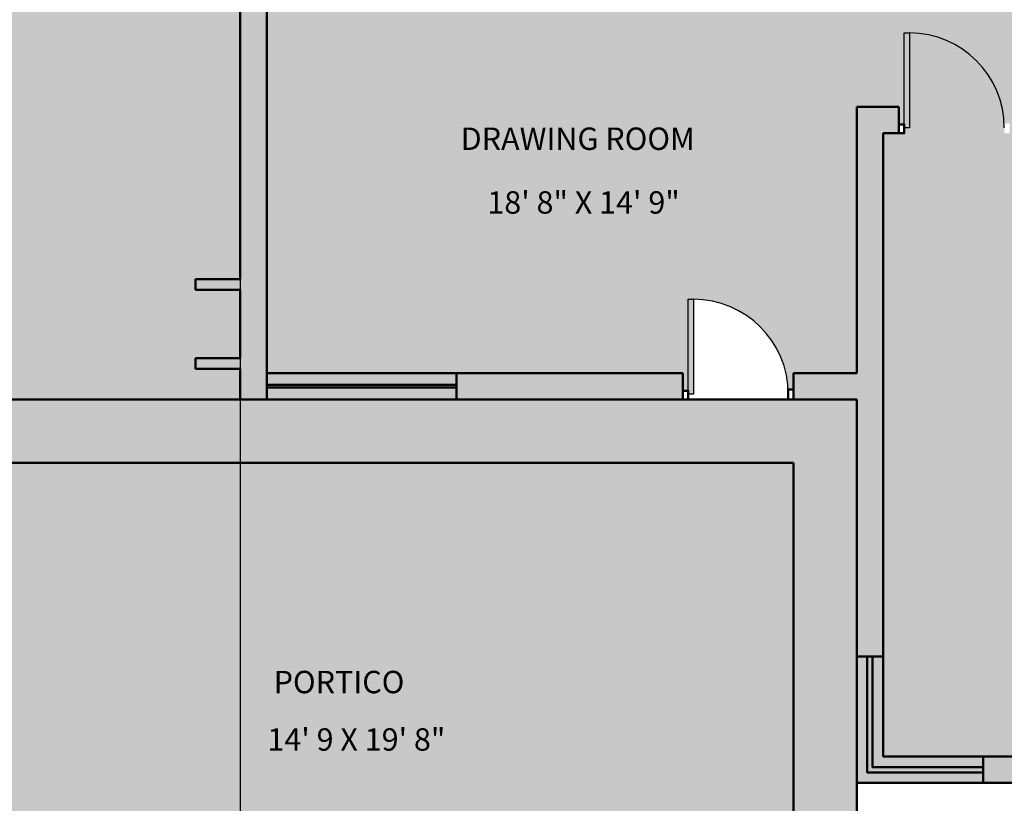
# Model space of a CAD drawing. Units: inches. Extents: x 925 to 2834, y 111 to 1355.
# Tile 3 of 25: x 1116 to 1490, y 377 to 675. Entities that reach past the tile are written whole.
import ezdxf

# ---------------------------------------------------------------- set-up
doc = ezdxf.new("R2010")
doc.units = ezdxf.units.IN
doc.header["$MEASUREMENT"] = 0
for name, color, linetype, lineweight in [('A-ANNO-DIMS', 2, 'Continuous', 18), ('A-AREA-IDEN', 7, 'Continuous', 18), ('A-DOOR', 2, 'Continuous', 25), ('A-FLOR-PATT', 252, 'Continuous', 13), ('A-WALL', 7, 'Continuous', 50), ('A-WALL-PATT', 8, 'Continuous', 13)]:
    doc.layers.add(name, color=color, linetype=linetype, lineweight=lineweight)
doc.styles.get("Standard").update_dxf_attribs({"font": 'arial.ttf'})
doc.dimstyles.get("Standard").update_dxf_attribs({"dimtxt": 6, "dimasz": 3, "dimexe": 0.18, "dimexo": 0.0625, "dimgap": 0.09, "dimtad": 0, "dimtih": 1, "dimtoh": 1, "dimdec": 1, "dimzin": 0, "dimdsep": 46, "dimlunit": 3, "dimtxsty": 'Standard', "dimblk": 'ARCHTICK', "dimcen": 0.09, "dimadec": 0, "dimazin": 0, "dimtfac": 1, "dimtdec": 1, "dimtofl": 0, "dimtmove": 0, "dimatfit": 3, "dimfxl": 1, "dimtolj": 1, "dimtzin": 0, "dimarcsym": 0})

# ---------------------------------------------------------------- blocks, each defined once
blk = doc.blocks.new('DOOR-900')
for p, q in [((0, 0), (0, 36)), ((0, 36), (2, 36)), ((2, 36), (2, 0)), ((2, 0), (0, 0))]:
    blk.add_line(p, q)
blk.add_arc((2, 0), 36, 0, 90)
blk = doc.blocks.new('_ArchTick')
at = {"color": 0, "linetype": 'ByBlock', "const_width": 0.15}
blk.add_lwpolyline([(-0.5, -0.5), (0.5, 0.5)], dxfattribs=at)
blk = doc.blocks.new('*D25')
at = {"layer": 'A-ANNO-DIMS', "color": 0, "lineweight": -2, "transparency": 16777216}
for p, q in [((1200.21, 727.53), (1200.21, 115.18)), ((1084.71, 265.03), (1084.71, 115.18)), ((1084.71, 115.36), (1132.51, 115.36)), ((1200.21, 115.36), (1152.42, 115.36))]:
    blk.add_line(p, q, dxfattribs=at)
at = {"layer": 'Defpoints', "color": 0, "transparency": 16777216}
for p in [(1200.21, 727.59), (1084.71, 265.09), (1200.21, 115.36)]:
    blk.add_point(p, dxfattribs=at)
at = {"layer": 'A-ANNO-DIMS', "color": 0, "lineweight": -2, "transparency": 16777216, "xscale": 3, "yscale": 3, "zscale": 3, "rotation": 180}
blk.add_blockref('_ArchTick', (1084.71, 115.36), dxfattribs=at)
at = {"layer": 'A-ANNO-DIMS', "color": 0, "lineweight": -2, "transparency": 16777216, "xscale": 3, "yscale": 3, "zscale": 3}
blk.add_blockref('_ArchTick', (1200.21, 115.36), dxfattribs=at)
at = {"layer": 'A-ANNO-DIMS', "color": 0, "transparency": 16777216, "insert": (1142.46, 115.36), "char_height": 6, "attachment_point": 5}
blk.add_mtext('\\A1;115.5', dxfattribs=at)
blk = doc.blocks.new('*D26')
at = {"layer": 'A-ANNO-DIMS', "color": 0, "lineweight": -2, "transparency": 16777216}
for p, q in [((1200.21, 727.53), (1200.21, 115.18)), ((1434.21, 385.03), (1434.21, 115.18)), ((1200.21, 115.36), (1310.46, 115.36)), ((1434.21, 115.36), (1323.97, 115.36))]:
    blk.add_line(p, q, dxfattribs=at)
at = {"layer": 'Defpoints', "color": 0, "transparency": 16777216}
for p in [(1200.21, 727.59), (1434.21, 385.09), (1434.21, 115.36)]:
    blk.add_point(p, dxfattribs=at)
at = {"layer": 'A-ANNO-DIMS', "color": 0, "lineweight": -2, "transparency": 16777216, "xscale": 3, "yscale": 3, "zscale": 3, "rotation": 180}
blk.add_blockref('_ArchTick', (1200.21, 115.36), dxfattribs=at)
at = {"layer": 'A-ANNO-DIMS', "color": 0, "lineweight": -2, "transparency": 16777216, "xscale": 3, "yscale": 3, "zscale": 3}
blk.add_blockref('_ArchTick', (1434.21, 115.36), dxfattribs=at)
at = {"layer": 'A-ANNO-DIMS', "color": 0, "transparency": 16777216, "insert": (1317.21, 115.36), "char_height": 6, "attachment_point": 5}
blk.add_mtext('\\A1;234', dxfattribs=at)
blk = doc.blocks.new('*D27')
at = {"layer": 'A-ANNO-DIMS', "color": 0, "lineweight": -2, "transparency": 16777216}
for p, q in [((1621.21, 395.03), (1621.21, 115.18)), ((1434.21, 385.03), (1434.21, 115.18)), ((1434.21, 115.36), (1521.28, 115.36)), ((1621.21, 115.36), (1534.15, 115.36))]:
    blk.add_line(p, q, dxfattribs=at)
at = {"layer": 'Defpoints', "color": 0, "transparency": 16777216}
for p in [(1621.21, 395.09), (1434.21, 385.09), (1621.21, 115.36)]:
    blk.add_point(p, dxfattribs=at)
at = {"layer": 'A-ANNO-DIMS', "color": 0, "lineweight": -2, "transparency": 16777216, "xscale": 3, "yscale": 3, "zscale": 3, "rotation": 180}
blk.add_blockref('_ArchTick', (1434.21, 115.36), dxfattribs=at)
at = {"layer": 'A-ANNO-DIMS', "color": 0, "lineweight": -2, "transparency": 16777216, "xscale": 3, "yscale": 3, "zscale": 3}
blk.add_blockref('_ArchTick', (1621.21, 115.36), dxfattribs=at)
at = {"layer": 'A-ANNO-DIMS', "color": 0, "transparency": 16777216, "insert": (1527.71, 115.36), "char_height": 6, "attachment_point": 5}
blk.add_mtext('\\A1;187', dxfattribs=at)

msp = doc.modelspace()

# ---------------------------------------------------------------- hatches: boundary and pattern name
at = {"layer": 'A-FLOR-PATT', "transparency": 33554605}
h = msp.add_hatch(color=256, dxfattribs=at)
h.dxf.hatch_style = 1
h.paths.add_polyline_path([(1931.688, 1294.5638), (991.7375, 1294.5638), (991.7375, 172.1134), (1931.688, 172.1134)])
h.paths.add_polyline_path([(1910.7128, 1273.5886), (1910.7128, 193.0886), (1012.7128, 193.0886), (1012.7128, 1273.5886)], flags=16)
h.paths.add_polyline_path([(1850.7128, 1213.5886), (1850.7128, 253.0886), (1072.7128, 253.0886), (1072.7128, 1213.5886)], flags=0)
h.paths.add_polyline_path([(1838.7128, 1201.5886), (1838.7128, 265.0886), (1084.7128, 265.0886), (1084.7128, 530.5886), (1084.7128, 1201.5886)], flags=0)
h.paths.add_polyline_path([(1547.6758, 1155.7396), (1547.6758, 1119.115), (1513.0687, 1119.115), (1513.0687, 1155.7396)], flags=0)
h.paths.add_polyline_path([(1600.1067, 1154.9439), (1634.7139, 1154.9439), (1634.7139, 1119.115), (1600.1067, 1119.115)], flags=0)
h.paths.add_polyline_path([(1505.2502, 1144.5358), (1505.2502, 1119.115), (1470.643, 1119.115), (1470.643, 1144.5358)], flags=0)
h.paths.add_polyline_path([(1559.1357, 1141.0962), (1593.7428, 1141.0962), (1593.7428, 1119.115), (1559.1357, 1119.115)], flags=0)
h.paths.add_polyline_path([(1462.8966, 1154.9439), (1462.8966, 1119.115), (1428.2895, 1119.115), (1428.2895, 1154.9439)], flags=0)
h.paths.add_polyline_path([(1642.4603, 1144.5358), (1677.0675, 1144.5358), (1677.0675, 1119.115), (1642.4603, 1119.115)], flags=0)
h.paths.add_polyline_path([(1422.3508, 1141.0962), (1422.3508, 1119.115), (1387.7436, 1119.115), (1387.7436, 1141.0962)], flags=0)
h.paths.add_polyline_path([(1684.8859, 1155.7396), (1719.4931, 1155.7396), (1719.4931, 1119.115), (1684.8859, 1119.115)], flags=0)
h.paths.add_polyline_path([(1718.7128, 1081.5886), (1718.7128, 1050.1249), (1715.7128, 1050.1249), (1715.7128, 1026.1249), (1715.7128, 1002.1249), (1718.7128, 1002.1249), (1730.7128, 1002.1249), (1730.7128, 998.1249), (1730.7128, 990.1249), (1730.7128, 986.1249), (1718.7128, 986.1249), (1718.7128, 893.5886), (1715.3735, 893.5886), (1715.3735, 891.5886), (1713.3735, 891.5886, 0.41421356), (1677.3735, 855.5886), (1713.3735, 855.5886), (1713.3735, 853.5886), (1715.3735, 853.5886), (1715.3735, 851.5886), (1718.7128, 851.5886), (1718.7128, 821.5865), (1734.4655, 821.5865), (1734.3735, 819.5886, -0.41421356), (1712.4415, 793.5886), (1712.4415, 791.5886), (1718.7128, 791.5886), (1718.7128, 717.5886), (1718.7128, 669.5886), (1732.7128, 669.5886), (1732.7128, 665.5886), (1732.7128, 641.5886), (1732.7128, 634.5886), (1732.7128, 610.5886), (1732.7128, 603.5886), (1718.7128, 603.5886), (1718.7128, 385.0886), (1434.2128, 385.0886), (1434.2128, 530.5886), (1410.2128, 530.5886), (1408.2128, 530.5886), (1408.2128, 532.5886, 0.41421356), (1372.2128, 568.5886), (1372.2128, 532.5886), (1370.2128, 532.5886), (1370.2128, 530.5886), (1368.2128, 530.5886), (1282.2128, 530.5886), (1210.2128, 530.5886), (1200.2128, 530.5886), (1200.2128, 542.1915), (1183.2307, 542.1915), (1183.2307, 546.1915), (1200.2128, 546.1915), (1200.2128, 572.1915), (1183.2307, 572.1915), (1183.2307, 576.1915), (1200.2128, 576.1915), (1200.2128, 727.5886), (1210.2128, 727.5886), (1234.2128, 727.5886), (1259.7128, 727.5886), (1259.7128, 775.5886), (1259.7128, 799.5886), (1259.7128, 847.5886), (1259.7128, 993.5872), (1259.7128, 1065.5872), (1259.7128, 1071.5886), (1219.6318, 1071.5886), (1219.6318, 1081.5886), (1084.7128, 1081.5886), (1084.7128, 1119.115), (1256.8974, 1119.115), (1256.8974, 1154.9439), (1291.5046, 1154.9439), (1291.5046, 1119.115), (1256.8974, 1119.115), (1256.6723, 1081.5886), (1293.7128, 1081.5886), (1341.7128, 1081.5886), (1341.7128, 1093.5886), (1347.7128, 1093.5886), (1371.7128, 1093.5886), (1377.7128, 1093.5886), (1377.7128, 1081.5886), (1668.7128, 1081.5886), (1668.7128, 1117.5886), (1675.7128, 1117.5886), (1711.7128, 1117.5886), (1718.7128, 1117.5886)], flags=0)
h.paths.add_polyline_path([(1376.2838, 1155.7396), (1376.2838, 1119.115), (1341.6766, 1119.115), (1341.6766, 1155.7396)], flags=0)
h.paths.add_polyline_path([(1341.7128, 1076.0886), (1293.7128, 1076.0886), (1293.7128, 1071.5886), (1269.7128, 1071.5886), (1269.7128, 1065.5872), (1266.7128, 1065.5872), (1266.7128, 1029.5872), (1265.7128, 1029.5872), (1265.7128, 993.5872), (1269.7128, 993.5872), (1269.7128, 903.5886), (1269.7128, 893.5886), (1269.7128, 847.5886), (1265.2128, 847.5886), (1265.2128, 799.5886), (1269.7128, 799.5886), (1269.7128, 775.5886), (1265.2128, 775.5886), (1265.2128, 727.5886), (1269.7128, 727.5886), (1444.2128, 727.5886), (1444.2128, 717.5886), (1234.2128, 717.5886), (1234.2128, 722.0886), (1210.2128, 722.0886), (1210.2128, 717.5886), (1210.2128, 540.5886), (1210.2128, 536.0886), (1282.2128, 536.0886), (1282.2128, 535.0886), (1210.2128, 535.0886), (1210.2128, 540.5886), (1210.2128, 717.5886), (1210.2128, 723.0886), (1234.2128, 723.0886), (1234.2128, 717.5886), (1444.2128, 717.5886), (1444.2128, 727.5886), (1269.7128, 727.5886), (1264.2128, 727.5886), (1264.2128, 775.5886), (1269.7128, 775.5886), (1269.7128, 799.5886), (1264.2128, 799.5886), (1264.2128, 847.5886), (1269.7128, 847.5886), (1269.7128, 893.5886), (1269.7128, 903.5886), (1269.7128, 993.5872), (1264.7128, 993.5872), (1264.7128, 1029.5872), (1265.7128, 1029.5872), (1265.7128, 1065.5872), (1269.7128, 1065.5872), (1269.7128, 1071.5886), (1293.7128, 1071.5886), (1293.7128, 1077.0886), (1341.7128, 1077.0886)], flags=0)
h.paths.add_polyline_path([(1730.9529, 1141.0962), (1765.5601, 1141.0962), (1765.5601, 1119.115), (1730.9529, 1119.115)], flags=0)
h.paths.add_polyline_path([(1333.8582, 1144.5358), (1333.8582, 1119.115), (1299.251, 1119.115), (1299.251, 1144.5358)], flags=0)
h.paths.add_polyline_path([(1592.7128, 968.5886), (1596.0342, 968.5886), (1602.7128, 968.5886), (1708.7128, 968.5886), (1708.7128, 903.5886), (1602.7128, 903.5886), (1602.7128, 938.5886), (1592.7128, 938.5886), (1592.7128, 903.5886), (1451.7128, 903.5886), (1451.7128, 893.5886), (1511.7128, 893.5886), (1511.7128, 881.5886), (1515.2128, 881.5886), (1518.7128, 881.5886), (1518.7128, 893.5886), (1592.7128, 893.5886), (1592.7128, 799.5886), (1518.7128, 799.5886), (1518.7128, 857.5886), (1511.7128, 857.5886), (1511.7128, 799.5886), (1511.7128, 772.0886), (1521.7128, 772.0886), (1521.7128, 792.5886), (1592.7128, 792.5886), (1592.7128, 727.5886), (1521.7128, 727.5886), (1521.7128, 748.0886), (1511.7128, 748.0886), (1511.7128, 717.5886), (1708.7128, 717.5886), (1714.2128, 717.5886), (1714.2128, 669.5886), (1708.7128, 669.5886), (1708.7128, 641.5886), (1492.2128, 641.5886), (1492.2128, 631.5886), (1621.2128, 631.5886), (1621.2128, 443.0886), (1625.7128, 443.0886), (1625.7128, 503.0886), (1625.7128, 507.5886), (1625.7128, 631.5886), (1708.7128, 631.5886), (1708.7128, 507.5886), (1655.7128, 507.5886), (1655.7128, 503.0886), (1708.7128, 503.0886), (1708.7128, 395.0886), (1625.7128, 395.0886), (1625.7128, 419.0886), (1621.2128, 419.0886), (1621.2128, 395.0886), (1482.2128, 395.0886), (1482.2128, 385.0886), (1434.2128, 385.0886), (1434.2128, 433.0886), (1444.2128, 433.0886), (1444.2128, 631.5886), (1450.2128, 631.5886), (1450.2128, 634.91), (1452.2128, 634.91), (1452.2128, 669.5886), (1454.2128, 669.5886, -0.40021217), (1490.1712, 635.3173), (1492.2128, 635.3173), (1492.2128, 641.5886), (1564.7128, 641.5886), (1564.7128, 677.5886), (1672.7128, 677.5886), (1672.7128, 681.5886), (1564.7128, 681.5886), (1564.7128, 717.5886), (1511.7128, 717.5886), (1511.7128, 748.0886), (1511.7128, 772.0886), (1511.7128, 799.5886), (1511.7128, 857.5886), (1511.8913, 857.5886), (1511.8913, 859.5886), (1515.6201, 859.5886, 0.41421356), (1537.552, 879.5886), (1513.552, 879.5886), (1511.8913, 879.5886), (1511.8913, 881.5886), (1511.7128, 881.5886), (1511.7128, 893.5886), (1451.7128, 893.5886), (1451.7128, 903.5886), (1592.7128, 903.5886), (1592.7128, 938.5886), (1592.7128, 940.5886), (1596.4415, 940.5886, 0.41421356), (1618.3735, 966.5886), (1594.3735, 966.5886), (1592.7128, 966.5886)], flags=0)
h.paths.add_polyline_path([(1377.7128, 903.5886), (1377.7128, 893.5886), (1305.7128, 893.5886), (1305.7128, 903.5886)], flags=0)
h.paths.add_polyline_path([(1708.7128, 821.5886), (1712.0342, 821.5886), (1712.0342, 819.5886), (1710.3735, 819.5886), (1708.7128, 819.5886)], flags=0)
h.paths.add_polyline_path([(1576.7128, 695.1992), (1575.5896, 693.6649), (1575.9687, 694.6994), (1575.4438, 695.1992), (1575.9687, 695.699), (1575.5896, 696.7335)], flags=0)
h.paths.add_polyline_path([(1565.9817, 662.3134), (1565.4568, 661.8136), (1565.8359, 660.7791), (1564.7128, 662.3134), (1565.8359, 663.8477), (1565.4568, 662.8132)], flags=0)
h.paths.add_polyline_path([(1444.2128, 433.0886), (1444.2128, 395.0886), (1482.2128, 395.0886), (1482.2128, 389.0886), (1438.2128, 389.0886), (1438.2128, 391.8608), (1438.2128, 433.0886)], flags=0)
h.paths.add_polyline_path([(1410.2128, 506.5886), (1410.2128, 289.0886), (1108.7128, 289.0886), (1108.7128, 506.5886)], flags=0)
h.paths.add_polyline_path([(1612.3153, 838.3016), (1680.4151, 838.3016), (1680.4151, 851.3131), (1612.3153, 851.3131)], flags=8)
h.paths.add_polyline_path([(1208.3174, 395.0436), (1282.1017, 395.0436), (1282.1017, 408.0552), (1208.3174, 408.0552)], flags=8)
h.paths.add_polyline_path([(1291.8049, 598.7427), (1369.8017, 598.7427), (1369.8017, 611.7542), (1291.8049, 611.7542)], flags=8)
h.paths.add_polyline_path([(1119.679, 917.3022), (1191.0817, 917.3022), (1191.0817, 930.3137), (1119.679, 930.3137)], flags=8)
h.paths.add_polyline_path([(1332.2261, 815.9808), (1410.2258, 815.9808), (1410.2258, 829.001), (1332.2261, 829.001)], flags=8)
h.paths.add_polyline_path([(1390.9013, 955.8158), (1475.4981, 955.8158), (1475.4981, 968.8273), (1390.9013, 968.8273)], flags=8)
h.paths.add_polyline_path([(1620.3436, 998.9325), (1688.4434, 998.9325), (1688.4434, 1011.944), (1620.3436, 1011.944)], flags=8)
h.paths.add_polyline_path([(1620.3436, 914.1039), (1691.7405, 914.1039), (1691.7405, 927.1155), (1620.3436, 927.1155)], flags=8)
h.paths.add_polyline_path([(1521.4542, 816.005), (1589.5569, 816.005), (1589.5569, 829.0253), (1521.4542, 829.0253)], flags=8)
h.paths.add_polyline_path([(1528.524, 740.3497), (1602.3082, 740.3497), (1602.3082, 753.3613), (1528.524, 753.3613)], flags=8)
h.paths.add_polyline_path([(1627.6094, 762.6128), (1702.3091, 762.6128), (1702.3091, 775.6244), (1627.6094, 775.6244)], flags=8)
h.paths.add_polyline_path([(1610.5442, 657.2751), (1684.3284, 657.2751), (1684.3284, 670.2867), (1610.5442, 670.2867)], flags=8)
h.paths.add_polyline_path([(1636.6983, 519.472), (1711.3981, 519.472), (1711.3981, 532.4835), (1636.6983, 532.4835)], flags=8)
h.paths.add_polyline_path([(1616.8577, 424.8539), (1694.8545, 424.8539), (1694.8545, 437.8654), (1616.8577, 437.8654)], flags=8)
h.paths.add_polyline_path([(1506.1456, 460.8838), (1579.9299, 460.8838), (1579.9299, 473.8953), (1506.1456, 473.8953)], flags=8)
h.paths.add_polyline_path([(1624.6119, 784.6011), (1696.9185, 784.6011), (1696.9185, 797.7864), (1624.6119, 797.7864)], flags=8)
h.paths.add_polyline_path([(1606.3732, 854.2194), (1683.3039, 854.2194), (1683.3039, 867.4048), (1606.3732, 867.4048)], flags=8)
h.paths.add_polyline_path([(1127.8008, 940.3581), (1165.1637, 940.3581), (1165.1637, 953.5348), (1127.8008, 953.5348)], flags=8)
h.paths.add_polyline_path([(1620.8657, 1019.4968), (1677.3447, 1019.4968), (1677.3447, 1032.6735), (1620.8657, 1032.6735)], flags=8)
h.paths.add_polyline_path([(1620.8643, 930.1821), (1703.0564, 930.1821), (1703.0564, 943.3675), (1620.8643, 943.3675)], flags=8)
h.paths.add_polyline_path([(1324.5702, 836.8338), (1408.0892, 836.8338), (1408.0892, 850.0191), (1324.5702, 850.0191)], flags=8)
h.paths.add_polyline_path([(1281.6584, 622.8885), (1383.6213, 622.8885), (1383.6213, 636.0739), (1281.6584, 636.0739)], flags=8)
h.paths.add_polyline_path([(1210.6721, 416.7893), (1269.1299, 416.7893), (1269.1299, 429.9747), (1210.6721, 429.9747)], flags=8)
h.paths.add_polyline_path([(1507.8264, 477.4836), (1586.7329, 477.4836), (1586.7329, 490.669), (1507.8264, 490.669)], flags=8)
h.paths.add_polyline_path([(1643.6238, 443.8135), (1696.6696, 443.8135), (1696.6696, 456.5643), (1643.6238, 456.5643)], flags=8)
h.paths.add_polyline_path([(1647.2466, 540.5638), (1693.1825, 540.5638), (1693.1825, 553.7491), (1647.2466, 553.7491)], flags=8)
h.paths.add_polyline_path([(1626.0633, 668.5064), (1673.3174, 668.5064), (1673.3174, 681.6831), (1626.0633, 681.6831)], flags=8)
h.paths.add_polyline_path([(1538.2915, 830.7872), (1567.5942, 830.7872), (1567.5942, 843.5293), (1538.2915, 843.5293)], flags=8)
h.paths.add_polyline_path([(1530.9338, 754.0477), (1559.576, 754.0477), (1559.576, 766.7898), (1530.9338, 766.7898)], flags=8)
h.paths.add_polyline_path([(1351.2461, 979.2309), (1513.8919, 979.2309), (1513.8919, 992.4076), (1351.2461, 992.4076)], flags=8)
at = {"layer": 'A-FLOR-PATT'}
h = msp.add_hatch(color=256, dxfattribs=at)
h.dxf.hatch_style = 1
h.paths.add_polyline_path([(1850.7128, 1213.5886), (1072.7128, 1213.5886), (1072.7128, 253.0886), (1850.7128, 253.0886)])
h.paths.add_polyline_path([(1084.7128, 1201.5886), (1838.7128, 1201.5886), (1838.7128, 265.0886), (1084.7128, 265.0886)], flags=16)
h.paths.add_polyline_path([(1183.2307, 576.1915), (1200.2128, 576.1915), (1200.2128, 727.5886), (1210.2128, 727.5886), (1234.2128, 727.5886), (1259.7128, 727.5886), (1259.7128, 775.5886), (1259.7128, 799.5886), (1259.7128, 847.5886), (1259.7128, 993.5872), (1259.7128, 1065.5872), (1259.7128, 1071.5886), (1219.6318, 1071.5886), (1219.6318, 1081.5886), (1293.7128, 1081.5886), (1341.7128, 1081.5886), (1341.7128, 1093.5886), (1347.7128, 1093.5886), (1347.7128, 1081.5886), (1371.7128, 1081.5886), (1371.7128, 1093.5886), (1377.7128, 1093.5886), (1377.7128, 1081.5886), (1668.7128, 1081.5886), (1668.7128, 1117.5886), (1675.7128, 1117.5886), (1675.7128, 1081.5886), (1711.7128, 1081.5886), (1711.7128, 1117.5886), (1718.7128, 1117.5886), (1718.7128, 1081.5886), (1718.7128, 1050.1249), (1715.7128, 1050.1249), (1715.7128, 1026.1249), (1715.7128, 1002.1249), (1718.7128, 1002.1249), (1730.7128, 1002.1249), (1730.7128, 998.1249), (1730.7128, 990.1249), (1730.7128, 986.1249), (1718.7128, 986.1249), (1718.7128, 893.5886), (1715.3735, 893.5886), (1715.3735, 891.5886), (1713.3735, 891.5886, 0.41421356), (1677.3735, 855.5886), (1713.3735, 855.5886), (1713.3735, 853.5886), (1715.3735, 853.5886), (1715.3735, 851.5886), (1718.7128, 851.5886), (1718.7128, 821.5865), (1734.4655, 821.5865), (1734.3735, 819.5886, -0.41421356), (1712.4415, 793.5886), (1712.4415, 791.5886), (1718.7128, 791.5886), (1718.7128, 717.5886), (1718.7128, 669.5886), (1732.7128, 669.5886), (1732.7128, 665.5886), (1732.7128, 641.5886), (1732.7128, 634.5886), (1732.7128, 610.5886), (1732.7128, 603.5886), (1718.7128, 603.5886), (1718.7128, 385.0886), (1434.2128, 385.0886), (1434.2128, 433.0886), (1434.2128, 530.5886), (1410.2128, 530.5886), (1408.2128, 530.5886), (1408.2128, 532.5886, 0.41421356), (1372.2128, 568.5886), (1372.2128, 532.5886), (1370.2128, 532.5886), (1370.2128, 530.5886), (1368.2128, 530.5886), (1282.2128, 530.5886), (1210.2128, 530.5886), (1200.2128, 530.5886), (1200.2128, 542.1915), (1183.2307, 542.1915), (1183.2307, 546.1915), (1200.2128, 546.1915), (1200.2128, 572.1915), (1183.2307, 572.1915)], flags=0)
h.paths.add_polyline_path([(1210.2128, 717.5886), (1210.2128, 723.0886), (1234.2128, 723.0886), (1234.2128, 717.5886), (1444.2128, 717.5886), (1444.2128, 727.5886), (1269.7128, 727.5886), (1264.2128, 727.5886), (1264.2128, 775.5886), (1269.7128, 775.5886), (1269.7128, 799.5886), (1264.2128, 799.5886), (1264.2128, 847.5886), (1269.7128, 847.5886), (1269.7128, 893.5886), (1269.7128, 903.5886), (1269.7128, 993.5872), (1264.7128, 993.5872), (1264.7128, 1029.5872), (1265.7128, 1029.5872), (1265.7128, 1065.5872), (1269.7128, 1065.5872), (1269.7128, 1071.5886), (1293.7128, 1071.5886), (1293.7128, 1077.0886), (1341.7128, 1077.0886), (1341.7128, 1076.0886), (1293.7128, 1076.0886), (1293.7128, 1071.5886), (1269.7128, 1071.5886), (1269.7128, 1065.5872), (1266.7128, 1065.5872), (1266.7128, 1029.5872), (1265.7128, 1029.5872), (1265.7128, 993.5872), (1269.7128, 993.5872), (1269.7128, 903.5886), (1269.7128, 893.5886), (1269.7128, 847.5886), (1265.2128, 847.5886), (1265.2128, 799.5886), (1269.7128, 799.5886), (1269.7128, 775.5886), (1265.2128, 775.5886), (1265.2128, 727.5886), (1269.7128, 727.5886), (1444.2128, 727.5886), (1444.2128, 717.5886), (1234.2128, 717.5886), (1234.2128, 722.0886), (1210.2128, 722.0886), (1210.2128, 717.5886), (1210.2128, 540.5886), (1210.2128, 536.0886), (1282.2128, 536.0886), (1282.2128, 535.0886), (1210.2128, 535.0886), (1210.2128, 540.5886)], flags=0)
h.paths.add_polyline_path([(1450.2128, 634.91), (1452.2128, 634.91), (1452.2128, 669.5886), (1454.2128, 669.5886, -0.40021217), (1490.1712, 635.3173), (1492.2128, 635.3173), (1492.2128, 641.5886), (1564.7128, 641.5886), (1564.7128, 677.5886), (1672.7128, 677.5886), (1672.7128, 681.5886), (1564.7128, 681.5886), (1564.7128, 717.5886), (1511.7128, 717.5886), (1511.7128, 748.0886), (1511.7128, 772.0886), (1511.7128, 799.5886), (1511.7128, 857.5886), (1511.8913, 857.5886), (1511.8913, 859.5886), (1515.6201, 859.5886, 0.41421356), (1537.552, 879.5886), (1513.552, 879.5886), (1511.8913, 879.5886), (1511.8913, 881.5886), (1511.7128, 881.5886), (1511.7128, 893.5886), (1451.7128, 893.5886), (1451.7128, 903.5886), (1592.7128, 903.5886), (1592.7128, 938.5886), (1592.7128, 940.5886), (1596.4415, 940.5886, 0.41421356), (1618.3735, 966.5886), (1594.3735, 966.5886), (1592.7128, 966.5886), (1592.7128, 968.5886), (1596.0342, 968.5886), (1602.7128, 968.5886), (1708.7128, 968.5886), (1708.7128, 903.5886), (1602.7128, 903.5886), (1602.7128, 938.5886), (1592.7128, 938.5886), (1592.7128, 903.5886), (1451.7128, 903.5886), (1451.7128, 893.5886), (1511.7128, 893.5886), (1511.7128, 881.5886), (1518.7128, 881.5886), (1518.7128, 893.5886), (1592.7128, 893.5886), (1592.7128, 799.5886), (1518.7128, 799.5886), (1518.7128, 857.5886), (1511.7128, 857.5886), (1511.7128, 799.5886), (1511.7128, 772.0886), (1521.7128, 772.0886), (1521.7128, 792.5886), (1592.7128, 792.5886), (1592.7128, 727.5886), (1521.7128, 727.5886), (1521.7128, 748.0886), (1511.7128, 748.0886), (1511.7128, 717.5886), (1708.7128, 717.5886), (1714.2128, 717.5886), (1714.2128, 669.5886), (1708.7128, 669.5886), (1708.7128, 641.5886), (1492.2128, 641.5886), (1492.2128, 631.5886), (1621.2128, 631.5886), (1621.2128, 443.0886), (1625.7128, 443.0886), (1625.7128, 503.0886), (1625.7128, 507.5886), (1625.7128, 631.5886), (1708.7128, 631.5886), (1708.7128, 507.5886), (1655.7128, 507.5886), (1655.7128, 503.0886), (1708.7128, 503.0886), (1708.7128, 395.0886), (1625.7128, 395.0886), (1625.7128, 419.0886), (1621.2128, 419.0886), (1621.2128, 395.0886), (1482.2128, 395.0886), (1482.2128, 389.0886), (1438.2128, 389.0886), (1438.2128, 391.8608), (1438.2128, 433.0886), (1444.2128, 433.0886), (1444.2128, 631.5886), (1450.2128, 631.5886)], flags=0)
h.paths.add_polyline_path([(1444.2128, 433.0886), (1444.2128, 395.0886), (1482.2128, 395.0886), (1482.2128, 391.0886), (1440.2128, 391.0886), (1440.2128, 391.8608), (1440.2128, 433.0886)], flags=0)
h.paths.add_polyline_path([(1305.7128, 893.5886), (1305.7128, 903.5886), (1377.7128, 903.5886), (1377.7128, 893.5886)], flags=0)
h.paths.add_polyline_path([(1564.7128, 662.3134), (1565.8359, 663.8477), (1565.4568, 662.8132), (1565.9817, 662.3134), (1565.4568, 661.8136), (1565.8359, 660.7791)], flags=0)
h.paths.add_polyline_path([(1575.4438, 695.1992), (1575.9687, 695.699), (1575.5896, 696.7335), (1576.7128, 695.1992), (1575.5896, 693.6649), (1575.9687, 694.6994)], flags=0)
h.paths.add_polyline_path([(1708.7128, 821.5886), (1712.0342, 821.5886), (1712.0342, 819.5886), (1710.3735, 819.5886), (1708.7128, 819.5886)], flags=0)
h = msp.add_hatch(color=256, dxfattribs=at)
h.dxf.hatch_style = 1
h.paths.add_polyline_path([(1718.7128, 603.5886), (1708.7128, 603.5886), (1708.7128, 507.5886), (1655.7128, 507.5886), (1655.7128, 503.0886), (1708.7128, 503.0886), (1708.7128, 395.0886), (1625.7128, 395.0886), (1625.7128, 419.0886), (1621.2128, 419.0886), (1621.2128, 395.0886), (1482.2128, 395.0886), (1482.2128, 385.0886), (1718.7128, 385.0886)])
h.paths.add_polyline_path([(1625.7128, 631.5886), (1708.7128, 631.5886), (1708.7128, 603.5886), (1718.7128, 603.5886), (1732.7128, 603.5886), (1732.7128, 610.5886), (1715.7128, 610.5886), (1715.7128, 634.5886), (1732.7128, 634.5886), (1732.7128, 641.5886), (1715.7128, 641.5886), (1715.7128, 665.5886), (1732.7128, 665.5886), (1732.7128, 669.5886), (1708.7128, 669.5886), (1708.7128, 641.5886), (1492.2128, 641.5886), (1492.2128, 631.5886), (1621.2128, 631.5886), (1621.2128, 443.0886), (1625.7128, 443.0886), (1625.7128, 503.0886), (1625.7128, 507.5886)])
h.paths.add_polyline_path([(1718.7128, 851.5886), (1708.7128, 851.5886), (1708.7128, 828.5886), (1602.7128, 828.5886), (1602.7128, 893.5886), (1708.7128, 893.5886), (1718.7128, 893.5886), (1718.7128, 986.1249), (1730.7128, 986.1249), (1730.7128, 990.1249), (1718.7128, 990.1249), (1718.7128, 998.1249), (1730.7128, 998.1249), (1730.7128, 1002.1249), (1718.7128, 1002.1249), (1708.7128, 1002.1249), (1708.7128, 975.5886), (1602.7128, 975.5886), (1602.7128, 1011.5886), (1592.7128, 1011.5886), (1592.7128, 968.5886), (1596.0342, 968.5886), (1602.7128, 968.5886), (1708.7128, 968.5886), (1708.7128, 903.5886), (1602.7128, 903.5886), (1602.7128, 938.5886), (1592.7128, 938.5886), (1592.7128, 903.5886), (1451.7128, 903.5886), (1451.7128, 893.5886), (1511.7128, 893.5886), (1511.7128, 881.5886), (1515.2128, 881.5886), (1518.7128, 881.5886), (1518.7128, 893.5886), (1592.7128, 893.5886), (1592.7128, 799.5886), (1518.7128, 799.5886), (1518.7128, 857.5886), (1511.7128, 857.5886), (1511.7128, 799.5886), (1511.7128, 772.0886), (1521.7128, 772.0886), (1521.7128, 792.5886), (1592.7128, 792.5886), (1592.7128, 727.5886), (1521.7128, 727.5886), (1521.7128, 748.0886), (1511.7128, 748.0886), (1511.7128, 717.5886), (1708.7128, 717.5886), (1718.7128, 717.5886), (1718.7128, 727.5886), (1718.7128, 791.5886), (1708.7128, 791.5886), (1708.7128, 727.5886), (1602.7128, 727.5886), (1602.7128, 821.5886), (1708.7128, 821.5886), (1712.0342, 821.5886), (1718.7128, 821.5886)])
h.paths.add_polyline_path([(1718.7128, 1081.5886), (1718.7128, 1117.5886), (1711.7128, 1117.5886), (1711.7128, 1081.5886), (1675.7128, 1081.5886), (1675.7128, 1117.5886), (1668.7128, 1117.5886), (1668.7128, 1081.5886), (1377.7128, 1081.5886), (1377.7128, 1093.5886), (1371.7128, 1093.5886), (1371.7128, 1081.5886), (1347.7128, 1081.5886), (1347.7128, 1093.5886), (1341.7128, 1093.5886), (1341.7128, 1081.5886), (1341.7128, 1071.5886), (1592.7128, 1071.5886), (1592.7128, 1035.5886), (1602.7128, 1035.5886), (1602.7128, 1071.5886), (1708.7128, 1071.5886), (1708.7128, 1050.1249), (1718.7128, 1050.1249)])
h.paths.add_polyline_path([(1293.7128, 1081.5886), (1219.6318, 1081.5886), (1219.6318, 1071.5886), (1259.7128, 1071.5886), (1259.7128, 1065.5872), (1269.7128, 1065.5872), (1269.7128, 1071.5886), (1293.7128, 1071.5886)])
h.paths.add_polyline_path([(1269.7128, 903.5886), (1269.7128, 993.5872), (1259.7128, 993.5872), (1259.7128, 847.5886), (1269.7128, 847.5886), (1269.7128, 893.5886)])
h.paths.add_polyline_path([(1377.7128, 903.5886), (1305.7128, 903.5886), (1305.7128, 893.5886), (1377.7128, 893.5886)])
h.paths.add_polyline_path([(1444.2128, 727.5886), (1269.7128, 727.5886), (1259.7128, 727.5886), (1234.2128, 727.5886), (1234.2128, 717.5886), (1444.2128, 717.5886)])
h.paths.add_polyline_path([(1269.7128, 799.5886), (1259.7128, 799.5886), (1259.7128, 775.5886), (1269.7128, 775.5886)])
h.paths.add_polyline_path([(1444.2128, 631.5886), (1450.2128, 631.5886), (1450.2128, 634.91), (1450.2128, 641.5886), (1434.2128, 641.5886), (1434.2128, 540.5886), (1410.2128, 540.5886), (1410.2128, 530.5886), (1434.2128, 530.5886), (1434.2128, 433.0886), (1444.2128, 433.0886)])
h.paths.add_polyline_path([(1368.2128, 533.91), (1368.2128, 540.5886), (1282.2128, 540.5886), (1282.2128, 530.5886), (1368.2128, 530.5886)])
h.paths.add_polyline_path([(1210.2128, 717.5886), (1210.2128, 727.5886), (1200.2128, 727.5886), (1200.2128, 576.1915), (1183.2307, 576.1915), (1183.2307, 572.1915), (1200.2128, 572.1915), (1200.2128, 546.1915), (1183.2307, 546.1915), (1183.2307, 542.1915), (1200.2128, 542.1915), (1200.2128, 530.5886), (1210.2128, 530.5886), (1210.2128, 540.5886)])
at = {"layer": 'A-FLOR-PATT', "transparency": 33554605}
h = msp.add_hatch(color=256, dxfattribs=at)
h.dxf.hatch_style = 1
h.paths.add_polyline_path([(1592.7128, 938.5886), (1592.7128, 940.5886), (1596.4415, 940.5886, 0.41421356), (1618.3735, 966.5886), (1594.3735, 966.5886), (1592.7128, 966.5886), (1592.7128, 968.5886), (1592.7128, 1011.5886), (1602.7128, 1011.5886), (1602.7128, 975.5886), (1708.7128, 975.5886), (1708.7128, 1002.1249), (1711.7128, 1002.1249), (1711.7128, 1026.1249), (1711.7128, 1050.1249), (1708.7128, 1050.1249), (1708.7128, 1071.5886), (1602.7128, 1071.5886), (1602.7128, 1035.5886), (1592.7128, 1035.5886), (1592.7128, 1071.5886), (1341.7128, 1071.5886), (1293.7128, 1071.5886), (1269.7128, 1071.5886), (1269.7128, 1065.5872), (1269.7128, 993.5872), (1269.7128, 903.5886), (1269.7128, 893.5886), (1269.7128, 847.5886), (1269.7128, 799.5886), (1269.7128, 775.5886), (1269.7128, 727.5886), (1444.2128, 727.5886), (1444.2128, 717.5886), (1234.2128, 717.5886), (1210.2128, 717.5886), (1210.2128, 540.5886), (1282.2128, 540.5886), (1368.2128, 540.5886), (1368.2128, 533.91), (1370.2128, 533.91), (1370.2128, 568.5886), (1372.2128, 568.5886, -0.40021217), (1408.1712, 534.3173), (1410.2128, 534.3173), (1410.2128, 540.5886), (1434.2128, 540.5886), (1434.2128, 641.5886), (1450.2128, 641.5886), (1450.2128, 634.91), (1452.2128, 634.91), (1452.2128, 669.5886), (1454.2128, 669.5886, -0.40021217), (1490.1712, 635.3173), (1492.2128, 635.3173), (1492.2128, 641.5886), (1564.7128, 641.5886), (1564.7128, 677.5886), (1672.7128, 677.5886), (1672.7128, 681.5886), (1564.7128, 681.5886), (1564.7128, 717.5886), (1511.7128, 717.5886), (1511.7128, 748.0886), (1511.7128, 772.0886), (1511.7128, 799.5886), (1511.7128, 857.5886), (1511.8913, 857.5886), (1511.8913, 859.5886), (1515.6201, 859.5886, 0.41421356), (1537.552, 879.5886), (1513.552, 879.5886), (1511.8913, 879.5886), (1511.8913, 881.5886), (1511.7128, 881.5886), (1511.7128, 893.5886), (1451.7128, 893.5886), (1451.7128, 903.5886), (1592.7128, 903.5886)])
h.paths.add_polyline_path([(1377.7128, 903.5886), (1377.7128, 893.5886), (1305.7128, 893.5886), (1305.7128, 903.5886)], flags=16)
h.paths.add_polyline_path([(1592.7128, 893.5886), (1518.7128, 893.5886), (1518.7128, 881.5865), (1537.6441, 881.5865), (1537.552, 879.5886, -0.41421356), (1515.6201, 859.5886), (1515.6201, 857.5886), (1518.7128, 857.5886), (1518.7128, 799.5886), (1592.7128, 799.5886)], flags=17)
h.paths.add_polyline_path([(1291.8049, 598.7427), (1369.8017, 598.7427), (1369.8017, 611.7542), (1291.8049, 611.7542)], flags=24)
h.paths.add_polyline_path([(1332.2261, 815.9808), (1410.2258, 815.9808), (1410.2258, 829.001), (1332.2261, 829.001)], flags=24)
h.paths.add_polyline_path([(1390.9013, 955.8158), (1475.4981, 955.8158), (1475.4981, 968.8273), (1390.9013, 968.8273)], flags=24)
h.paths.add_polyline_path([(1620.3436, 998.9325), (1688.4434, 998.9325), (1688.4434, 1011.944), (1620.3436, 1011.944)], flags=24)
h.paths.add_polyline_path([(1620.8657, 1019.4968), (1677.3447, 1019.4968), (1677.3447, 1032.6735), (1620.8657, 1032.6735)], flags=24)
h.paths.add_polyline_path([(1324.5702, 836.8338), (1408.0892, 836.8338), (1408.0892, 850.0191), (1324.5702, 850.0191)], flags=24)
h.paths.add_polyline_path([(1281.6584, 622.8885), (1383.6213, 622.8885), (1383.6213, 636.0739), (1281.6584, 636.0739)], flags=24)
h.paths.add_polyline_path([(1626.0633, 668.5064), (1673.3174, 668.5064), (1673.3174, 681.6831), (1626.0633, 681.6831)], flags=25)
h.paths.add_polyline_path([(1351.2461, 979.2309), (1513.8919, 979.2309), (1513.8919, 992.4076), (1351.2461, 992.4076)], flags=24)
h.paths.add_polyline_path([(1521.4542, 816.005), (1589.5569, 816.005), (1589.5569, 829.0253), (1521.4542, 829.0253)], flags=24)
h.paths.add_polyline_path([(1538.2915, 830.7872), (1567.5942, 830.7872), (1567.5942, 843.5293), (1538.2915, 843.5293)], flags=24)
h.paths.add_polyline_path([(1636.6983, 519.472), (1711.3981, 519.472), (1711.3981, 532.4835), (1636.6983, 532.4835)], flags=9)
h.paths.add_polyline_path([(1616.8577, 424.8539), (1694.8545, 424.8539), (1694.8545, 437.8654), (1616.8577, 437.8654)], flags=9)
h.paths.add_polyline_path([(1506.1456, 460.8838), (1579.9299, 460.8838), (1579.9299, 473.8953), (1506.1456, 473.8953)], flags=9)
h.paths.add_polyline_path([(1606.3732, 854.2194), (1683.3039, 854.2194), (1683.3039, 867.4048), (1606.3732, 867.4048)], flags=25)
h.paths.add_polyline_path([(1507.8264, 477.4836), (1586.7329, 477.4836), (1586.7329, 490.669), (1507.8264, 490.669)], flags=9)
h.paths.add_polyline_path([(1643.6238, 443.8135), (1696.6696, 443.8135), (1696.6696, 456.5643), (1643.6238, 456.5643)], flags=9)
h.paths.add_polyline_path([(1647.2466, 540.5638), (1693.1825, 540.5638), (1693.1825, 553.7491), (1647.2466, 553.7491)], flags=25)
h = msp.add_hatch(color=256, dxfattribs=at)
h.dxf.hatch_style = 1
h.paths.add_polyline_path([(1200.2128, 727.5886), (1084.7128, 727.5886), (1084.7128, 530.5886), (1200.2128, 530.5886), (1200.2128, 542.1915), (1183.2307, 542.1915), (1183.2307, 546.1915), (1200.2128, 546.1915), (1200.2128, 572.1915), (1183.2307, 572.1915), (1183.2307, 576.1915), (1200.2128, 576.1915)])
h.paths.add_polyline_path([(1612.3153, 838.3016), (1680.4151, 838.3016), (1680.4151, 851.3131), (1612.3153, 851.3131)], flags=9)
h.paths.add_polyline_path([(1291.8049, 598.7427), (1369.8017, 598.7427), (1369.8017, 611.7542), (1291.8049, 611.7542)], flags=9)
h.paths.add_polyline_path([(1119.679, 917.3022), (1191.0817, 917.3022), (1191.0817, 930.3137), (1119.679, 930.3137)], flags=9)
h.paths.add_polyline_path([(1332.2261, 815.9808), (1410.2258, 815.9808), (1410.2258, 829.001), (1332.2261, 829.001)], flags=9)
h.paths.add_polyline_path([(1390.9013, 955.8158), (1475.4981, 955.8158), (1475.4981, 968.8273), (1390.9013, 968.8273)], flags=9)
h.paths.add_polyline_path([(1620.3436, 998.9325), (1688.4434, 998.9325), (1688.4434, 1011.944), (1620.3436, 1011.944)], flags=9)
h.paths.add_polyline_path([(1620.3436, 914.1039), (1691.7405, 914.1039), (1691.7405, 927.1155), (1620.3436, 927.1155)], flags=9)
h.paths.add_polyline_path([(1521.4542, 816.005), (1589.5569, 816.005), (1589.5569, 829.0253), (1521.4542, 829.0253)], flags=9)
h.paths.add_polyline_path([(1522.4337, 740.3497), (1596.218, 740.3497), (1596.218, 753.3613), (1522.4337, 753.3613)], flags=9)
h.paths.add_polyline_path([(1606.3732, 854.2194), (1683.3039, 854.2194), (1683.3039, 867.4048), (1606.3732, 867.4048)], flags=9)
h.paths.add_polyline_path([(1127.8008, 940.3581), (1165.1637, 940.3581), (1165.1637, 953.5348), (1127.8008, 953.5348)], flags=9)
h.paths.add_polyline_path([(1620.8657, 1019.4968), (1677.3447, 1019.4968), (1677.3447, 1032.6735), (1620.8657, 1032.6735)], flags=9)
h.paths.add_polyline_path([(1620.8643, 930.1821), (1703.0564, 930.1821), (1703.0564, 943.3675), (1620.8643, 943.3675)], flags=9)
h.paths.add_polyline_path([(1324.5702, 836.8338), (1408.0892, 836.8338), (1408.0892, 850.0191), (1324.5702, 850.0191)], flags=9)
h.paths.add_polyline_path([(1281.6584, 622.8885), (1383.6213, 622.8885), (1383.6213, 636.0739), (1281.6584, 636.0739)], flags=9)
h.paths.add_polyline_path([(1626.0633, 668.5064), (1673.3174, 668.5064), (1673.3174, 681.6831), (1626.0633, 681.6831)], flags=9)
h.paths.add_polyline_path([(1538.2915, 830.7872), (1567.5942, 830.7872), (1567.5942, 843.5293), (1538.2915, 843.5293)], flags=9)
h.paths.add_polyline_path([(1351.2461, 979.2309), (1513.8919, 979.2309), (1513.8919, 992.4076), (1351.2461, 992.4076)], flags=9)
h = msp.add_hatch(color=256, dxfattribs=at)
h.dxf.hatch_style = 1
h.paths.add_polyline_path([(1621.2128, 631.5886), (1492.2128, 631.5886), (1490.2128, 631.5886), (1490.2128, 633.5886, 0.41421356), (1454.2128, 669.5886), (1454.2128, 633.5886), (1452.2128, 633.5886), (1452.2128, 631.5886), (1450.2128, 631.5886), (1444.2128, 631.5886), (1444.2128, 395.0886), (1482.2128, 395.0886), (1621.2128, 395.0886), (1621.2128, 419.0886), (1625.7128, 419.0886), (1625.7128, 395.0886), (1708.7128, 395.0886), (1708.7128, 503.0886), (1655.7128, 503.0886), (1655.7128, 507.5886), (1708.7128, 507.5886), (1708.7128, 631.5886), (1625.7128, 631.5886), (1625.7128, 507.5886), (1625.7128, 503.0886), (1625.7128, 443.0886), (1621.2128, 443.0886)])
h.paths.add_polyline_path([(1636.6983, 519.472), (1711.3981, 519.472), (1711.3981, 532.4835), (1636.6983, 532.4835)], flags=9)
h.paths.add_polyline_path([(1616.8577, 424.8539), (1694.8545, 424.8539), (1694.8545, 437.8654), (1616.8577, 437.8654)], flags=24)
h.paths.add_polyline_path([(1506.1456, 460.8838), (1579.9299, 460.8838), (1579.9299, 473.8953), (1506.1456, 473.8953)], flags=24)
h.paths.add_polyline_path([(1507.8264, 477.4836), (1586.7329, 477.4836), (1586.7329, 490.669), (1507.8264, 490.669)], flags=24)
h.paths.add_polyline_path([(1643.6238, 443.8135), (1696.6696, 443.8135), (1696.6696, 456.5643), (1643.6238, 456.5643)], flags=24)
h.paths.add_polyline_path([(1647.2466, 540.5638), (1693.1825, 540.5638), (1693.1825, 553.7491), (1647.2466, 553.7491)], flags=24)
h.paths.add_polyline_path([(1612.3153, 838.3016), (1680.4151, 838.3016), (1680.4151, 851.3131), (1612.3153, 851.3131)], flags=9)
h.paths.add_polyline_path([(1291.8049, 598.7427), (1369.8017, 598.7427), (1369.8017, 611.7542), (1291.8049, 611.7542)], flags=9)
h.paths.add_polyline_path([(1119.679, 917.3022), (1191.0817, 917.3022), (1191.0817, 930.3137), (1119.679, 930.3137)], flags=9)
h.paths.add_polyline_path([(1332.2261, 815.9808), (1410.2258, 815.9808), (1410.2258, 829.001), (1332.2261, 829.001)], flags=9)
h.paths.add_polyline_path([(1390.9013, 955.8158), (1475.4981, 955.8158), (1475.4981, 968.8273), (1390.9013, 968.8273)], flags=9)
h.paths.add_polyline_path([(1620.3436, 998.9325), (1688.4434, 998.9325), (1688.4434, 1011.944), (1620.3436, 1011.944)], flags=9)
h.paths.add_polyline_path([(1620.3436, 914.1039), (1691.7405, 914.1039), (1691.7405, 927.1155), (1620.3436, 927.1155)], flags=9)
h.paths.add_polyline_path([(1521.4542, 816.005), (1589.5569, 816.005), (1589.5569, 829.0253), (1521.4542, 829.0253)], flags=9)
h.paths.add_polyline_path([(1528.524, 740.3497), (1602.3082, 740.3497), (1602.3082, 753.3613), (1528.524, 753.3613)], flags=9)
h.paths.add_polyline_path([(1627.6094, 762.6128), (1702.3091, 762.6128), (1702.3091, 775.6244), (1627.6094, 775.6244)], flags=9)
h.paths.add_polyline_path([(1624.6119, 784.6011), (1696.9185, 784.6011), (1696.9185, 797.7864), (1624.6119, 797.7864)], flags=9)
h.paths.add_polyline_path([(1606.3732, 854.2194), (1683.3039, 854.2194), (1683.3039, 867.4048), (1606.3732, 867.4048)], flags=9)
h.paths.add_polyline_path([(1127.8008, 940.3581), (1165.1637, 940.3581), (1165.1637, 953.5348), (1127.8008, 953.5348)], flags=9)
h.paths.add_polyline_path([(1620.8657, 1019.4968), (1677.3447, 1019.4968), (1677.3447, 1032.6735), (1620.8657, 1032.6735)], flags=9)
h.paths.add_polyline_path([(1620.8643, 930.1821), (1703.0564, 930.1821), (1703.0564, 943.3675), (1620.8643, 943.3675)], flags=9)
h.paths.add_polyline_path([(1324.5702, 836.8338), (1408.0892, 836.8338), (1408.0892, 850.0191), (1324.5702, 850.0191)], flags=9)
h.paths.add_polyline_path([(1281.6584, 622.8885), (1383.6213, 622.8885), (1383.6213, 636.0739), (1281.6584, 636.0739)], flags=9)
h.paths.add_polyline_path([(1626.0633, 668.5064), (1673.3174, 668.5064), (1673.3174, 681.6831), (1626.0633, 681.6831)], flags=9)
h.paths.add_polyline_path([(1538.2915, 830.7872), (1567.5942, 830.7872), (1567.5942, 843.5293), (1538.2915, 843.5293)], flags=9)
h.paths.add_polyline_path([(1530.9338, 754.0477), (1559.576, 754.0477), (1559.576, 766.7898), (1530.9338, 766.7898)], flags=9)
h.paths.add_polyline_path([(1351.2461, 979.2309), (1513.8919, 979.2309), (1513.8919, 992.4076), (1351.2461, 992.4076)], flags=9)
at = {"layer": 'A-FLOR-PATT'}
h = msp.add_hatch(color=256, dxfattribs=at)
h.dxf.hatch_style = 1
h.paths.add_polyline_path([(1713.3735, 855.5886), (1677.3735, 855.5886), (1677.3735, 853.5886), (1713.3735, 853.5886)])
h.paths.add_polyline_path([(1372.2128, 568.5886), (1370.2128, 568.5886), (1370.2128, 532.5886), (1372.2128, 532.5886)])
h.paths.add_polyline_path([(1734.4655, 821.5865), (1712.0342, 821.5865), (1712.0342, 819.5886), (1734.3735, 819.5886)])
h.paths.add_polyline_path([(1454.2128, 669.5886), (1452.2128, 669.5886), (1452.2128, 633.5886), (1454.2128, 633.5886)])
h.paths.add_polyline_path([(1537.6441, 881.5865), (1515.2128, 881.5865), (1515.2128, 879.5886), (1537.552, 879.5886)])
at = {"layer": 'A-FLOR-PATT', "transparency": 33554498}
h = msp.add_hatch(color=256, dxfattribs=at)
h.dxf.hatch_style = 1
h.paths.add_polyline_path([(1434.2128, 530.5886), (1084.7128, 530.5886), (1084.7128, 265.0886), (1434.2128, 265.0886)])
h.paths.add_polyline_path([(1410.2128, 506.5886), (1410.2128, 289.0886), (1108.7128, 289.0886), (1108.7128, 506.5886)], flags=16)
h.paths.add_polyline_path([(1410.2128, 506.5886), (1108.7128, 506.5886), (1108.7128, 289.0886), (1410.2128, 289.0886)], flags=16)
at = {"layer": 'A-FLOR-PATT'}
h = msp.add_hatch(color=256, dxfattribs=at)
h.dxf.hatch_style = 1
h.paths.add_polyline_path([(1482.2128, 395.0886), (1444.2128, 395.0886), (1444.2128, 433.0886), (1440.2128, 433.0886), (1440.2128, 391.8608), (1440.2128, 391.0886), (1482.2128, 391.0886)], flags=17)
h.paths.add_polyline_path([(1482.2128, 389.0886), (1438.2128, 389.0886), (1438.2128, 391.8608), (1438.2128, 433.0886), (1434.2128, 433.0886), (1434.2128, 385.0886), (1482.2128, 385.0886)])
h = msp.add_hatch(color=256, dxfattribs=at)
h.dxf.hatch_style = 1
h.paths.add_polyline_path([(1482.2128, 391.0886), (1440.2128, 391.0886), (1440.2128, 391.8608), (1440.2128, 433.0886), (1438.2128, 433.0886), (1438.2128, 391.8608), (1438.2128, 389.0886), (1482.2128, 389.0886)])
at = {"layer": 'A-WALL-PATT'}
h = msp.add_hatch(color=256, dxfattribs=at)
h.dxf.hatch_style = 1
h.paths.add_polyline_path([(1282.2128, 540.5886), (1210.2128, 540.5886), (1210.2128, 536.0886), (1282.2128, 536.0886)])
h.paths.add_polyline_path([(1282.2128, 535.0886), (1210.2128, 535.0886), (1210.2128, 530.5886), (1282.2128, 530.5886)])
h = msp.add_hatch(color=256, dxfattribs=at)
h.dxf.hatch_style = 1
h.paths.add_polyline_path([(1282.2128, 536.0886), (1210.2128, 536.0886), (1210.2128, 535.0886), (1282.2128, 535.0886)])

# ---------------------------------------------------------------- linework, layer by layer
at = {"layer": 'A-WALL'}
for p, q in [((1200.2128, 727.5886), (1200.2128, 576.1915)), ((1210.2128, 717.5886), (1210.2128, 540.5886)), ((1434.2128, 641.5886), (1434.2128, 540.5886)), ((1450.2128, 641.5886), (1434.2128, 641.5886)), ((1450.2128, 631.5886), (1450.2128, 641.5886)), ((1444.2128, 631.5886), (1444.2128, 395.0886)), ((1450.2128, 631.5886), (1444.2128, 631.5886)), ((1200.2128, 576.1915), (1183.2307, 576.1915)), ((1183.2307, 572.1915), (1183.2307, 576.1915)), ((1200.2128, 572.1915), (1183.2307, 572.1915)), ((1200.2128, 572.1915), (1200.2128, 546.1915)), ((1200.2128, 546.1915), (1183.2307, 546.1915)), ((1183.2307, 542.1915), (1183.2307, 546.1915)), ((1200.2128, 542.1915), (1183.2307, 542.1915)), ((1200.2128, 542.1915), (1200.2128, 530.5886)), ((1210.2128, 540.5886), (1210.2128, 530.5886)), ((1282.2128, 540.5886), (1282.2128, 530.5886)), ((1368.2128, 540.5886), (1282.2128, 540.5886)), ((1368.2128, 540.5886), (1368.2128, 530.5886)), ((1434.2128, 540.5886), (1410.2128, 540.5886)), ((1410.2128, 540.5886), (1410.2128, 530.5886)), ((1282.2128, 536.0886), (1210.2128, 536.0886)), ((1282.2128, 535.0886), (1210.2128, 535.0886)), ((1210.2128, 530.5886), (1200.2128, 530.5886)), ((1368.2128, 530.5886), (1282.2128, 530.5886)), ((1434.2128, 530.5886), (1410.2128, 530.5886)), ((1434.2128, 530.5886), (1434.2128, 385.0886)), ((1434.2128, 385.0886), (1434.2128, 530.5886)), ((1434.2128, 433.0886), (1444.2128, 433.0886)), ((1434.2128, 433.0886), (1434.2128, 385.0886)), ((1444.2128, 433.0886), (1434.2128, 433.0886)), ((1444.2128, 433.0886), (1444.2128, 395.0886)), ((1621.2128, 395.0886), (1444.2128, 395.0886)), ((1444.2128, 395.0886), (1482.2128, 395.0886)), ((1482.2128, 385.0886), (1482.2128, 395.0886)), ((1482.2128, 395.0886), (1482.2128, 385.0886)), ((1718.7128, 385.0886), (1434.2128, 385.0886)), ((1434.2128, 385.0886), (1482.2128, 385.0886)), ((1460.2128, 385.0886), (1434.2128, 385.0886)), ((1434.2128, 385.0886), (1434.2128, 265.0886)), ((1434.2128, 265.0886), (1434.2128, 385.0886)), ((1434.2128, 385.0886), (1714, 385.0886))]:
    msp.add_line(p, q, dxfattribs=at)
for points in [[(1450.2128, 634.91), (1452.2128, 634.91), (1452.2128, 631.5886), (1450.2128, 631.5886)], [(1282.2128, 530.5886), (1210.2128, 530.5886), (1210.2128, 540.5886), (1282.2128, 540.5886)], [(1368.2128, 533.91), (1370.2128, 533.91), (1370.2128, 530.5886), (1368.2128, 530.5886)], [(1408.2128, 534.3173), (1410.2128, 534.3173), (1410.2128, 530.5886), (1408.2128, 530.5886)], [(1434.2128, 530.5886), (1084.7128, 530.5886), (1084.7128, 265.0886), (1434.2128, 265.0886)], [(1410.2128, 506.5886), (1108.7128, 506.5886), (1108.7128, 289.0886), (1410.2128, 289.0886)]]:
    msp.add_lwpolyline(points, close=True, dxfattribs=at)
for points in [[(1482.2128, 389.0886), (1438.2128, 389.0886), (1438.2128, 391.8608), (1438.2128, 433.0886)], [(1482.2128, 391.0886), (1440.2128, 391.0886), (1440.2128, 391.8608), (1440.2128, 433.0886)]]:
    msp.add_lwpolyline(points, dxfattribs=at)

# ---------------------------------------------------------------- block references
at = {"layer": 'A-DOOR'}
for p in [(1452.213, 633.589), (1370.213, 532.589)]:
    msp.add_blockref('DOOR-900', p, dxfattribs=at)

# ---------------------------------------------------------------- texts
at = {"layer": 'A-AREA-IDEN'}
for s, height, p in [('DRAWING ROOM', 8.494735, (1283.856, 625.2309)), ('18\' 8" X 14\' 9"', 8.494735, (1293.9735, 601.0561)), ('PORTICO', 8.49473, (1212.8697, 419.1317)), ('14\' 9 X 19\' 8"', 8.494735, (1210.486, 397.3571))]:
    msp.add_text(s, height=height, dxfattribs=at).set_placement(p)

# ---------------------------------------------------------------- dimensions: what is measured, and where the dimension line sits
at = {"layer": 'A-ANNO-DIMS'}
for base, p1, p2, override, picture, middle in [((1200.2128, 115.3634), (1084.7128, 265.0886), (1200.2128, 727.5886), {"dimdec": 1, "dimlfac": 1, "dimrnd": 0, "dimzin": 0, "dimdsep": 46, "dimlunit": 2}, '*D25', (1142.4628, 115.3634)), ((1434.2128, 115.3634), (1200.2128, 727.5886), (1434.2128, 385.0886), {"dimdec": 0, "dimlfac": 1, "dimrnd": 0, "dimzin": 0, "dimdsep": 46, "dimlunit": 2}, '*D26', (1317.2128, 115.3634)), ((1621.2128, 115.3634), (1434.2128, 385.0886), (1621.2128, 395.0886), {"dimdec": 0, "dimlfac": 1, "dimrnd": 0, "dimzin": 0, "dimdsep": 46, "dimlunit": 2}, '*D27', (1527.7128, 115.3634))]:
    dim = msp.add_linear_dim(base=base, p1=p1, p2=p2, dimstyle='Standard', override=override, dxfattribs=at)
    dim.commit()
    dim.dimension.update_dxf_attribs({"geometry": picture, "text_midpoint": middle})

doc.saveas('drawing.dxf')
